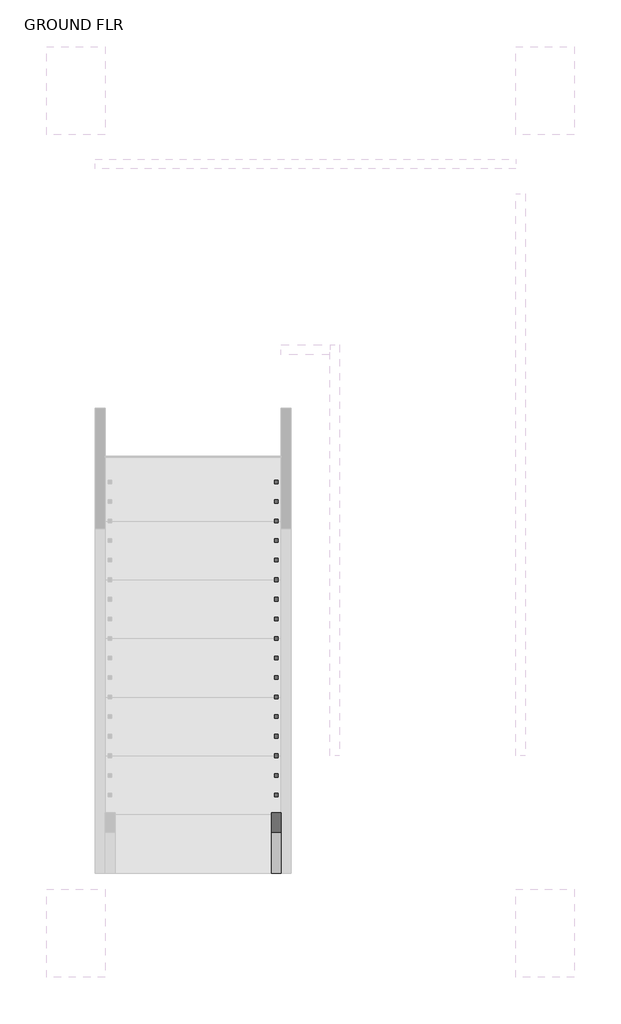
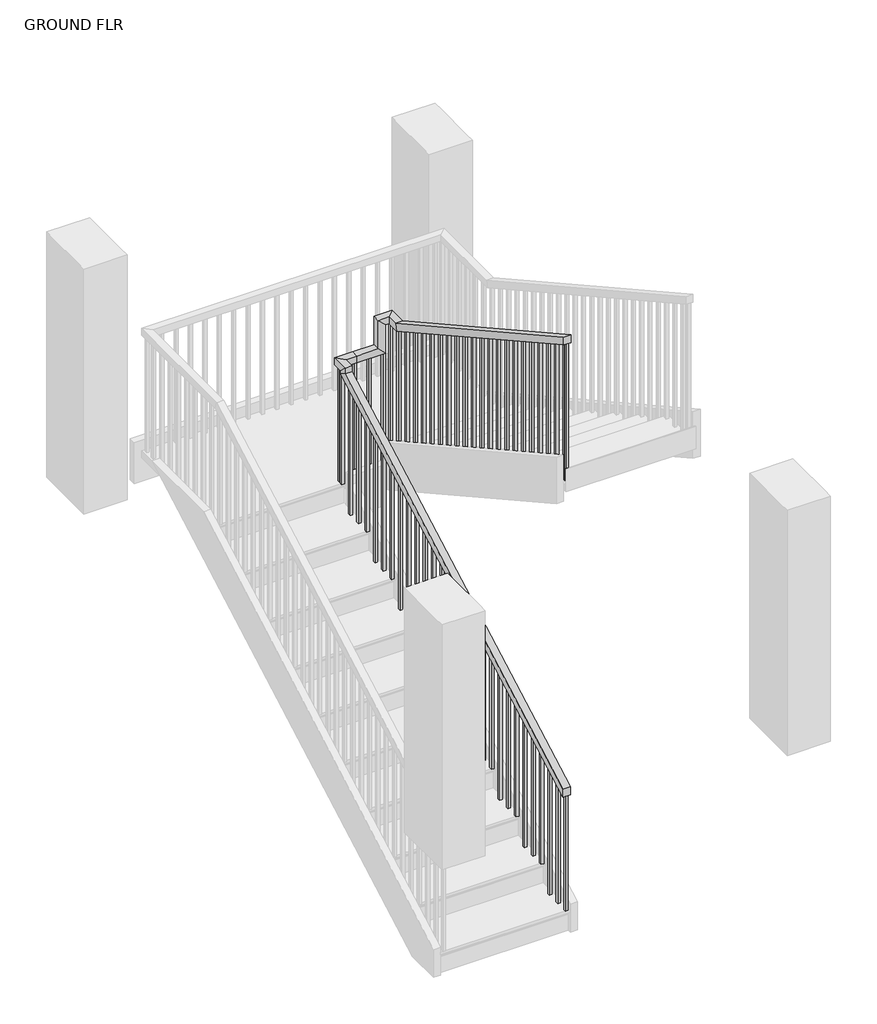
# One storey, part 3 of 4: 1 railing.
"""IFC4 building model written with IfcOpenShell, lengths in millimetres."""

from ifc_helpers import new_model, si_unit, frame, origin, place, context, project, spatial, polyline, outline, extrude, faceted_brep, element, save

model = new_model("IFC4")

# Units and contexts
model_context = context("Model", 3, world=origin())
ifc_project = project(units=[si_unit("LENGTHUNIT", "METRE", prefix="MILLI")], contexts=[model_context])

# Site, building, storey
site = spatial("IfcSite", under=ifc_project)
building = spatial("IfcBuilding", under=site)
storey = spatial("IfcBuildingStorey", under=building, Name="GROUND FLR", Elevation=304.8)

# Railing
placement = place(None, origin())
element("IfcRailing", 1, ObjectType="Handrail - Rectangular", at=placement, inside=storey, context=model_context, shape_type="SolidModel", body=[
    faceted_brep([(-128.5175798, -5516.2061634, 1388.5333333), (-128.5175798, -5516.2061634, 1330.420221), (-77.7175798, -5516.2061634, 1330.420221), (-77.7175798, -5516.2061634, 1388.5333333), (-128.5175798, -2849.2061634, 2870.2), (-128.5175798, -2798.4061634, 2840.3091099), (-77.7175798, -2798.4061634, 2840.3091099), (-77.7175798, -2849.2061634, 2870.2), (-128.5175798, -2849.2061634, 2912.5333333), (-128.5175798, -2798.4061634, 2861.7333333), (-77.7175798, -2798.4061634, 2861.7333333), (-77.7175798, -2849.2061634, 2912.5333333), (-128.5175798, -2722.2061634, 2912.5333333), (-128.5175798, -2722.2061634, 2861.7333333), (-77.7175798, -2773.0061634, 2861.7333333), (-77.7175798, -2773.0061634, 2912.5333333), (-1.5175798, -2722.2061634, 2912.5333333), (-1.5175798, -2722.2061634, 2861.7333333), (-1.5175798, -2773.0061634, 2861.7333333), (-1.5175798, -2773.0061634, 2912.5333333), (150.8824202, -2722.2061634, 2912.5333333), (201.6824202, -2722.2061634, 2861.7333333), (201.6824202, -2773.0061634, 2861.7333333), (150.8824202, -2773.0061634, 2912.5333333), (150.8824202, -2722.2061634, 3124.2), (201.6824202, -2722.2061634, 3073.4), (201.6824202, -2773.0061634, 3073.4), (150.8824202, -2773.0061634, 3124.2), (277.8824202, -2722.2061634, 3124.2), (277.8824202, -2722.2061634, 3073.4), (227.0824202, -2773.0061634, 3073.4), (227.0824202, -2773.0061634, 3124.2), (277.8824202, -2849.2061634, 3124.2), (277.8824202, -2862.3697656, 3073.4), (227.0824202, -2862.3697656, 3073.4), (227.0824202, -2849.2061634, 3124.2), (277.8824202, -4906.6061634, 4267.2), (227.0824202, -4906.6061634, 4267.2), (227.0824202, -4906.6061634, 4209.0868876), (277.8824202, -4906.6061634, 4209.0868876)], [[[0, 1, 2, 3]], [[1, 0, 4, 5]], [[2, 1, 5, 6]], [[3, 2, 6, 7]], [[0, 3, 7, 4]], [[5, 4, 8, 9]], [[6, 5, 9, 10]], [[7, 6, 10, 11]], [[4, 7, 11, 8]], [[9, 8, 12, 13]], [[10, 9, 13, 14]], [[11, 10, 14, 15]], [[8, 11, 15, 12]], [[13, 12, 16, 17]], [[14, 13, 17, 18]], [[15, 14, 18, 19]], [[12, 15, 19, 16]], [[17, 16, 20, 21]], [[18, 17, 21, 22]], [[19, 18, 22, 23]], [[16, 19, 23, 20]], [[21, 20, 24, 25]], [[22, 21, 25, 26]], [[23, 22, 26, 27]], [[20, 23, 27, 24]], [[25, 24, 28, 29]], [[26, 25, 29, 30]], [[27, 26, 30, 31]], [[24, 27, 31, 28]], [[29, 28, 32, 33]], [[30, 29, 33, 34]], [[31, 30, 34, 35]], [[28, 31, 35, 32]], [[36, 37, 38, 39]], [[33, 32, 36, 39]], [[34, 33, 39, 38]], [[35, 34, 38, 37]], [[32, 35, 37, 36]]]),
    extrude(outline(polyline([(-4890.7311634, 4200.2674432), (-4871.6811634, 4189.6841099), (-4871.6811634, 3183.4666667), (-4890.7311634, 3183.4666667), (-4890.7311634, 4200.2674432)])), frame((242.9574202, 0.0, 0.0), z_axis=(1.0, 0.0, 0.0), x_axis=(0.0, 1.0, 0.0)), (0.0, 0.0, 1.0), 19.05),
    extrude(outline(polyline([(-4789.1311634, 4143.8229988), (-4770.0811634, 4133.2396654), (-4770.0811634, 3183.4666667), (-4789.1311634, 3183.4666667), (-4789.1311634, 4143.8229988)])), frame((242.9574202, 0.0, 0.0), z_axis=(1.0, 0.0, 0.0), x_axis=(0.0, 1.0, 0.0)), (0.0, 0.0, 1.0), 19.05),
    extrude(outline(polyline([(-4687.5311634, 4087.3785543), (-4668.4811634, 4076.795221), (-4668.4811634, 3183.4666667), (-4687.5311634, 3183.4666667), (-4687.5311634, 4087.3785543)])), frame((242.9574202, 0.0, 0.0), z_axis=(1.0, 0.0, 0.0), x_axis=(0.0, 1.0, 0.0)), (0.0, 0.0, 1.0), 19.05),
    extrude(outline(polyline([(-4585.9311634, 4030.9341099), (-4566.8811634, 4020.3507765), (-4566.8811634, 3014.1333333), (-4585.9311634, 3014.1333333), (-4585.9311634, 4030.9341099)])), frame((242.9574202, 0.0, 0.0), z_axis=(1.0, 0.0, 0.0), x_axis=(0.0, 1.0, 0.0)), (0.0, 0.0, 1.0), 19.05),
    extrude(outline(polyline([(-4484.3311634, 3974.4896654), (-4465.2811634, 3963.9063321), (-4465.2811634, 3014.1333333), (-4484.3311634, 3014.1333333), (-4484.3311634, 3974.4896654)])), frame((242.9574202, 0.0, 0.0), z_axis=(1.0, 0.0, 0.0), x_axis=(0.0, 1.0, 0.0)), (0.0, 0.0, 1.0), 19.05),
    extrude(outline(polyline([(-4382.7311634, 3918.045221), (-4363.6811634, 3907.4618876), (-4363.6811634, 3014.1333333), (-4382.7311634, 3014.1333333), (-4382.7311634, 3918.045221)])), frame((242.9574202, 0.0, 0.0), z_axis=(1.0, 0.0, 0.0), x_axis=(0.0, 1.0, 0.0)), (0.0, 0.0, 1.0), 19.05),
    extrude(outline(polyline([(-4281.1311634, 3861.6007765), (-4262.0811634, 3851.0174432), (-4262.0811634, 2844.8), (-4281.1311634, 2844.8), (-4281.1311634, 3861.6007765)])), frame((242.9574202, 0.0, 0.0), z_axis=(1.0, 0.0, 0.0), x_axis=(0.0, 1.0, 0.0)), (0.0, 0.0, 1.0), 19.05),
    extrude(outline(polyline([(-4179.5311634, 3805.1563321), (-4160.4811634, 3794.5729988), (-4160.4811634, 2844.8), (-4179.5311634, 2844.8), (-4179.5311634, 3805.1563321)])), frame((242.9574202, 0.0, 0.0), z_axis=(1.0, 0.0, 0.0), x_axis=(0.0, 1.0, 0.0)), (0.0, 0.0, 1.0), 19.05),
    extrude(outline(polyline([(-4077.9311634, 3748.7118876), (-4058.8811634, 3738.1285543), (-4058.8811634, 2844.8), (-4077.9311634, 2844.8), (-4077.9311634, 3748.7118876)])), frame((242.9574202, 0.0, 0.0), z_axis=(1.0, 0.0, 0.0), x_axis=(0.0, 1.0, 0.0)), (0.0, 0.0, 1.0), 19.05),
    extrude(outline(polyline([(-3976.3311634, 3692.2674432), (-3957.2811634, 3681.6841099), (-3957.2811634, 2675.4666667), (-3976.3311634, 2675.4666667), (-3976.3311634, 3692.2674432)])), frame((242.9574202, 0.0, 0.0), z_axis=(1.0, 0.0, 0.0), x_axis=(0.0, 1.0, 0.0)), (0.0, 0.0, 1.0), 19.05),
    extrude(outline(polyline([(-3874.7311634, 3635.8229988), (-3855.6811634, 3625.2396654), (-3855.6811634, 2675.4666667), (-3874.7311634, 2675.4666667), (-3874.7311634, 3635.8229988)])), frame((242.9574202, 0.0, 0.0), z_axis=(1.0, 0.0, 0.0), x_axis=(0.0, 1.0, 0.0)), (0.0, 0.0, 1.0), 19.05),
    extrude(outline(polyline([(-3773.1311634, 3579.3785543), (-3754.0811634, 3568.795221), (-3754.0811634, 2675.4666667), (-3773.1311634, 2675.4666667), (-3773.1311634, 3579.3785543)])), frame((242.9574202, 0.0, 0.0), z_axis=(1.0, 0.0, 0.0), x_axis=(0.0, 1.0, 0.0)), (0.0, 0.0, 1.0), 19.05),
    extrude(outline(polyline([(-3671.5311634, 3522.9341099), (-3652.4811634, 3512.3507765), (-3652.4811634, 2506.1333333), (-3671.5311634, 2506.1333333), (-3671.5311634, 3522.9341099)])), frame((242.9574202, 0.0, 0.0), z_axis=(1.0, 0.0, 0.0), x_axis=(0.0, 1.0, 0.0)), (0.0, 0.0, 1.0), 19.05),
    extrude(outline(polyline([(-3569.9311634, 3466.4896654), (-3550.8811634, 3455.9063321), (-3550.8811634, 2506.1333333), (-3569.9311634, 2506.1333333), (-3569.9311634, 3466.4896654)])), frame((242.9574202, 0.0, 0.0), z_axis=(1.0, 0.0, 0.0), x_axis=(0.0, 1.0, 0.0)), (0.0, 0.0, 1.0), 19.05),
    extrude(outline(polyline([(-3468.3311634, 3410.045221), (-3449.2811634, 3399.4618876), (-3449.2811634, 2506.1333333), (-3468.3311634, 2506.1333333), (-3468.3311634, 3410.045221)])), frame((242.9574202, 0.0, 0.0), z_axis=(1.0, 0.0, 0.0), x_axis=(0.0, 1.0, 0.0)), (0.0, 0.0, 1.0), 19.05),
    extrude(outline(polyline([(-3366.7311634, 3353.6007765), (-3347.6811634, 3343.0174432), (-3347.6811634, 2336.8), (-3366.7311634, 2336.8), (-3366.7311634, 3353.6007765)])), frame((242.9574202, 0.0, 0.0), z_axis=(1.0, 0.0, 0.0), x_axis=(0.0, 1.0, 0.0)), (0.0, 0.0, 1.0), 19.05),
    extrude(outline(polyline([(-3265.1311634, 3297.1563321), (-3246.0811634, 3286.5729988), (-3246.0811634, 2336.8), (-3265.1311634, 2336.8), (-3265.1311634, 3297.1563321)])), frame((242.9574202, 0.0, 0.0), z_axis=(1.0, 0.0, 0.0), x_axis=(0.0, 1.0, 0.0)), (0.0, 0.0, 1.0), 19.05),
    extrude(outline(polyline([(-3163.5311634, 3240.7118876), (-3144.4811634, 3230.1285543), (-3144.4811634, 2336.8), (-3163.5311634, 2336.8), (-3163.5311634, 3240.7118876)])), frame((242.9574202, 0.0, 0.0), z_axis=(1.0, 0.0, 0.0), x_axis=(0.0, 1.0, 0.0)), (0.0, 0.0, 1.0), 19.05),
    extrude(outline(polyline([(-3061.9311634, 3184.2674432), (-3042.8811634, 3173.6841099), (-3042.8811634, 2167.4666667), (-3061.9311634, 2167.4666667), (-3061.9311634, 3184.2674432)])), frame((242.9574202, 0.0, 0.0), z_axis=(1.0, 0.0, 0.0), x_axis=(0.0, 1.0, 0.0)), (0.0, 0.0, 1.0), 19.05),
    extrude(outline(polyline([(-2960.3311634, 3127.8229988), (-2941.2811634, 3117.2396654), (-2941.2811634, 2167.4666667), (-2960.3311634, 2167.4666667), (-2960.3311634, 3127.8229988)])), frame((242.9574202, 0.0, 0.0), z_axis=(1.0, 0.0, 0.0), x_axis=(0.0, 1.0, 0.0)), (0.0, 0.0, 1.0), 19.05),
    extrude(outline(polyline([(-2858.7311634, 3071.3785543), (-2839.6811634, 3060.795221), (-2839.6811634, 2167.4666667), (-2858.7311634, 2167.4666667), (-2858.7311634, 3071.3785543)])), frame((242.9574202, 0.0, 0.0), z_axis=(1.0, 0.0, 0.0), x_axis=(0.0, 1.0, 0.0)), (0.0, 0.0, 1.0), 19.05),
    extrude(outline(polyline([(192.1574202, -2757.1311634), (192.1574202, -2738.0811634), (211.2074202, -2738.0811634), (211.2074202, -2757.1311634), (192.1574202, -2757.1311634)])), frame((0.0, 0.0, 1998.1333333), z_axis=(0.0, 0.0, 1.0), x_axis=(1.0, 0.0, 0.0)), (0.0, 0.0, 1.0), 1075.2666667),
    extrude(outline(polyline([(90.5574202, -2757.1311634), (90.5574202, -2738.0811634), (109.6074202, -2738.0811634), (109.6074202, -2757.1311634), (90.5574202, -2757.1311634)])), frame((0.0, 0.0, 1998.1333333), z_axis=(0.0, 0.0, 1.0), x_axis=(1.0, 0.0, 0.0)), (0.0, 0.0, 1.0), 863.6),
    extrude(outline(polyline([(-11.0425798, -2757.1311634), (-11.0425798, -2738.0811634), (8.0074202, -2738.0811634), (8.0074202, -2757.1311634), (-11.0425798, -2757.1311634)])), frame((0.0, 0.0, 1998.1333333), z_axis=(0.0, 0.0, 1.0), x_axis=(1.0, 0.0, 0.0)), (0.0, 0.0, 1.0), 863.6),
    extrude(outline(polyline([(-93.5925798, -2782.5311634), (-112.6425798, -2782.5311634), (-112.6425798, -2763.4811634), (-93.5925798, -2763.4811634), (-93.5925798, -2782.5311634)])), frame((0.0, 0.0, 1998.1333333), z_axis=(0.0, 0.0, 1.0), x_axis=(1.0, 0.0, 0.0)), (0.0, 0.0, 1.0), 863.6),
    extrude(outline(polyline([(-2884.1311634, 2792.6841099), (-2865.0811634, 2803.2674432), (-2865.0811634, 1828.8), (-2884.1311634, 1828.8), (-2884.1311634, 2792.6841099)])), frame((-112.6425798, 0.0, 0.0), z_axis=(1.0, 0.0, 0.0), x_axis=(0.0, 1.0, 0.0)), (0.0, 0.0, 1.0), 19.05),
    extrude(outline(polyline([(-2985.7311634, 2736.2396654), (-2966.6811634, 2746.8229988), (-2966.6811634, 1828.8), (-2985.7311634, 1828.8), (-2985.7311634, 2736.2396654)])), frame((-112.6425798, 0.0, 0.0), z_axis=(1.0, 0.0, 0.0), x_axis=(0.0, 1.0, 0.0)), (0.0, 0.0, 1.0), 19.05),
    extrude(outline(polyline([(-3087.3311634, 2679.795221), (-3068.2811634, 2690.3785543), (-3068.2811634, 1828.8), (-3087.3311634, 1828.8), (-3087.3311634, 2679.795221)])), frame((-112.6425798, 0.0, 0.0), z_axis=(1.0, 0.0, 0.0), x_axis=(0.0, 1.0, 0.0)), (0.0, 0.0, 1.0), 19.05),
    extrude(outline(polyline([(-3188.9311634, 2623.3507765), (-3169.8811634, 2633.9341099), (-3169.8811634, 1659.4666667), (-3188.9311634, 1659.4666667), (-3188.9311634, 2623.3507765)])), frame((-112.6425798, 0.0, 0.0), z_axis=(1.0, 0.0, 0.0), x_axis=(0.0, 1.0, 0.0)), (0.0, 0.0, 1.0), 19.05),
    extrude(outline(polyline([(-3290.5311634, 2566.9063321), (-3271.4811634, 2577.4896654), (-3271.4811634, 1659.4666667), (-3290.5311634, 1659.4666667), (-3290.5311634, 2566.9063321)])), frame((-112.6425798, 0.0, 0.0), z_axis=(1.0, 0.0, 0.0), x_axis=(0.0, 1.0, 0.0)), (0.0, 0.0, 1.0), 19.05),
    extrude(outline(polyline([(-3392.1311634, 2510.4618876), (-3373.0811634, 2521.045221), (-3373.0811634, 1659.4666667), (-3392.1311634, 1659.4666667), (-3392.1311634, 2510.4618876)])), frame((-112.6425798, 0.0, 0.0), z_axis=(1.0, 0.0, 0.0), x_axis=(0.0, 1.0, 0.0)), (0.0, 0.0, 1.0), 19.05),
    extrude(outline(polyline([(-3493.7311634, 2454.0174432), (-3474.6811634, 2464.6007765), (-3474.6811634, 1490.1333333), (-3493.7311634, 1490.1333333), (-3493.7311634, 2454.0174432)])), frame((-112.6425798, 0.0, 0.0), z_axis=(1.0, 0.0, 0.0), x_axis=(0.0, 1.0, 0.0)), (0.0, 0.0, 1.0), 19.05),
    extrude(outline(polyline([(-3595.3311634, 2397.5729988), (-3576.2811634, 2408.1563321), (-3576.2811634, 1490.1333333), (-3595.3311634, 1490.1333333), (-3595.3311634, 2397.5729988)])), frame((-112.6425798, 0.0, 0.0), z_axis=(1.0, 0.0, 0.0), x_axis=(0.0, 1.0, 0.0)), (0.0, 0.0, 1.0), 19.05),
    extrude(outline(polyline([(-3696.9311634, 2341.1285543), (-3677.8811634, 2351.7118876), (-3677.8811634, 1490.1333333), (-3696.9311634, 1490.1333333), (-3696.9311634, 2341.1285543)])), frame((-112.6425798, 0.0, 0.0), z_axis=(1.0, 0.0, 0.0), x_axis=(0.0, 1.0, 0.0)), (0.0, 0.0, 1.0), 19.05),
    extrude(outline(polyline([(-3798.5311634, 2284.6841099), (-3779.4811634, 2295.2674432), (-3779.4811634, 1320.8), (-3798.5311634, 1320.8), (-3798.5311634, 2284.6841099)])), frame((-112.6425798, 0.0, 0.0), z_axis=(1.0, 0.0, 0.0), x_axis=(0.0, 1.0, 0.0)), (0.0, 0.0, 1.0), 19.05),
    extrude(outline(polyline([(-3900.1311634, 2228.2396654), (-3881.0811634, 2238.8229988), (-3881.0811634, 1320.8), (-3900.1311634, 1320.8), (-3900.1311634, 2228.2396654)])), frame((-112.6425798, 0.0, 0.0), z_axis=(1.0, 0.0, 0.0), x_axis=(0.0, 1.0, 0.0)), (0.0, 0.0, 1.0), 19.05),
    extrude(outline(polyline([(-4001.7311634, 2171.795221), (-3982.6811634, 2182.3785543), (-3982.6811634, 1320.8), (-4001.7311634, 1320.8), (-4001.7311634, 2171.795221)])), frame((-112.6425798, 0.0, 0.0), z_axis=(1.0, 0.0, 0.0), x_axis=(0.0, 1.0, 0.0)), (0.0, 0.0, 1.0), 19.05),
    extrude(outline(polyline([(-4103.3311634, 2115.3507765), (-4084.2811634, 2125.9341099), (-4084.2811634, 1151.4666667), (-4103.3311634, 1151.4666667), (-4103.3311634, 2115.3507765)])), frame((-112.6425798, 0.0, 0.0), z_axis=(1.0, 0.0, 0.0), x_axis=(0.0, 1.0, 0.0)), (0.0, 0.0, 1.0), 19.05),
    extrude(outline(polyline([(-4204.9311634, 2058.9063321), (-4185.8811634, 2069.4896654), (-4185.8811634, 1151.4666667), (-4204.9311634, 1151.4666667), (-4204.9311634, 2058.9063321)])), frame((-112.6425798, 0.0, 0.0), z_axis=(1.0, 0.0, 0.0), x_axis=(0.0, 1.0, 0.0)), (0.0, 0.0, 1.0), 19.05),
    extrude(outline(polyline([(-4306.5311634, 2002.4618876), (-4287.4811634, 2013.045221), (-4287.4811634, 1151.4666667), (-4306.5311634, 1151.4666667), (-4306.5311634, 2002.4618876)])), frame((-112.6425798, 0.0, 0.0), z_axis=(1.0, 0.0, 0.0), x_axis=(0.0, 1.0, 0.0)), (0.0, 0.0, 1.0), 19.05),
    extrude(outline(polyline([(-4408.1311634, 1946.0174432), (-4389.0811634, 1956.6007765), (-4389.0811634, 982.1333333), (-4408.1311634, 982.1333333), (-4408.1311634, 1946.0174432)])), frame((-112.6425798, 0.0, 0.0), z_axis=(1.0, 0.0, 0.0), x_axis=(0.0, 1.0, 0.0)), (0.0, 0.0, 1.0), 19.05),
    extrude(outline(polyline([(-4509.7311634, 1889.5729988), (-4490.6811634, 1900.1563321), (-4490.6811634, 982.1333333), (-4509.7311634, 982.1333333), (-4509.7311634, 1889.5729988)])), frame((-112.6425798, 0.0, 0.0), z_axis=(1.0, 0.0, 0.0), x_axis=(0.0, 1.0, 0.0)), (0.0, 0.0, 1.0), 19.05),
    extrude(outline(polyline([(-4611.3311634, 1833.1285543), (-4592.2811634, 1843.7118876), (-4592.2811634, 982.1333333), (-4611.3311634, 982.1333333), (-4611.3311634, 1833.1285543)])), frame((-112.6425798, 0.0, 0.0), z_axis=(1.0, 0.0, 0.0), x_axis=(0.0, 1.0, 0.0)), (0.0, 0.0, 1.0), 19.05),
    extrude(outline(polyline([(-4712.9311634, 1776.6841099), (-4693.8811634, 1787.2674432), (-4693.8811634, 812.8), (-4712.9311634, 812.8), (-4712.9311634, 1776.6841099)])), frame((-112.6425798, 0.0, 0.0), z_axis=(1.0, 0.0, 0.0), x_axis=(0.0, 1.0, 0.0)), (0.0, 0.0, 1.0), 19.05),
    extrude(outline(polyline([(-4814.5311634, 1720.2396654), (-4795.4811634, 1730.8229988), (-4795.4811634, 812.8), (-4814.5311634, 812.8), (-4814.5311634, 1720.2396654)])), frame((-112.6425798, 0.0, 0.0), z_axis=(1.0, 0.0, 0.0), x_axis=(0.0, 1.0, 0.0)), (0.0, 0.0, 1.0), 19.05),
    extrude(outline(polyline([(-4916.1311634, 1663.795221), (-4897.0811634, 1674.3785543), (-4897.0811634, 812.8), (-4916.1311634, 812.8), (-4916.1311634, 1663.795221)])), frame((-112.6425798, 0.0, 0.0), z_axis=(1.0, 0.0, 0.0), x_axis=(0.0, 1.0, 0.0)), (0.0, 0.0, 1.0), 19.05),
    extrude(outline(polyline([(-5017.7311634, 1607.3507765), (-4998.6811634, 1617.9341099), (-4998.6811634, 643.4666667), (-5017.7311634, 643.4666667), (-5017.7311634, 1607.3507765)])), frame((-112.6425798, 0.0, 0.0), z_axis=(1.0, 0.0, 0.0), x_axis=(0.0, 1.0, 0.0)), (0.0, 0.0, 1.0), 19.05),
    extrude(outline(polyline([(-5119.3311634, 1550.9063321), (-5100.2811634, 1561.4896654), (-5100.2811634, 643.4666667), (-5119.3311634, 643.4666667), (-5119.3311634, 1550.9063321)])), frame((-112.6425798, 0.0, 0.0), z_axis=(1.0, 0.0, 0.0), x_axis=(0.0, 1.0, 0.0)), (0.0, 0.0, 1.0), 19.05),
    extrude(outline(polyline([(-5220.9311634, 1494.4618876), (-5201.8811634, 1505.045221), (-5201.8811634, 643.4666667), (-5220.9311634, 643.4666667), (-5220.9311634, 1494.4618876)])), frame((-112.6425798, 0.0, 0.0), z_axis=(1.0, 0.0, 0.0), x_axis=(0.0, 1.0, 0.0)), (0.0, 0.0, 1.0), 19.05),
    extrude(outline(polyline([(-5322.5311634, 1438.0174432), (-5303.4811634, 1448.6007765), (-5303.4811634, 474.1333333), (-5322.5311634, 474.1333333), (-5322.5311634, 1438.0174432)])), frame((-112.6425798, 0.0, 0.0), z_axis=(1.0, 0.0, 0.0), x_axis=(0.0, 1.0, 0.0)), (0.0, 0.0, 1.0), 19.05),
    extrude(outline(polyline([(-5424.1311634, 1381.5729988), (-5405.0811634, 1392.1563321), (-5405.0811634, 474.1333333), (-5424.1311634, 474.1333333), (-5424.1311634, 1381.5729988)])), frame((-112.6425798, 0.0, 0.0), z_axis=(1.0, 0.0, 0.0), x_axis=(0.0, 1.0, 0.0)), (0.0, 0.0, 1.0), 19.05),
    extrude(outline(polyline([(242.9574202, -2757.1311634), (242.9574202, -2738.0811634), (262.0074202, -2738.0811634), (262.0074202, -2757.1311634), (242.9574202, -2757.1311634)])), frame((0.0, 0.0, 1998.1333333), z_axis=(0.0, 0.0, 1.0), x_axis=(1.0, 0.0, 0.0)), (0.0, 0.0, 1.0), 1075.2666667),
    extrude(outline(polyline([(-93.5925798, -2757.1311634), (-112.6425798, -2757.1311634), (-112.6425798, -2738.0811634), (-93.5925798, -2738.0811634), (-93.5925798, -2757.1311634)])), frame((0.0, 0.0, 1998.1333333), z_axis=(0.0, 0.0, 1.0), x_axis=(1.0, 0.0, 0.0)), (0.0, 0.0, 1.0), 863.6),
    extrude(outline(polyline([(-4906.6061634, 4209.0868876), (-4887.5561634, 4198.5035543), (-4887.5561634, 3183.4666667), (-4906.6061634, 3183.4666667), (-4906.6061634, 4209.0868876)])), frame((242.9574202, 0.0, 0.0), z_axis=(1.0, 0.0, 0.0), x_axis=(0.0, 1.0, 0.0)), (0.0, 0.0, 1.0), 19.05),
    extrude(outline(polyline([(-5516.2061634, 1330.420221), (-5497.1561634, 1341.0035543), (-5497.1561634, 474.1333333), (-5516.2061634, 474.1333333), (-5516.2061634, 1330.420221)])), frame((-112.6425798, 0.0, 0.0), z_axis=(1.0, 0.0, 0.0), x_axis=(0.0, 1.0, 0.0)), (0.0, 0.0, 1.0), 19.05),
])

save(model, "model.ifc")

# Revit data of these elements
# Type "Handrail - Rectangular"
#   Assembly Code = "C2010400"
#   built-in parameter 1008612 = 0.0416667 (stored number, unit not read)
#   built-in parameter 1008611 = 0.0416667 (stored number, unit not read)
#   built-in parameter 1008609 = 0.333333 (stored number, unit not read)
#   built-in parameter 1008604 = 0.166667 (stored number, unit not read)
#   built-in parameter 1008603 = 0.166667 (stored number, unit not read)
#   Railing Height = 3' - 0"
#   built-in parameter 1008630 = 2
#   built-in parameter 1008610 = 2
#   built-in parameter 1008618 = Baluster - Square : 3/4"
# Element 1 (IfcRailing, "Handrail - Rectangular")
#   Phase Created = New Construction
